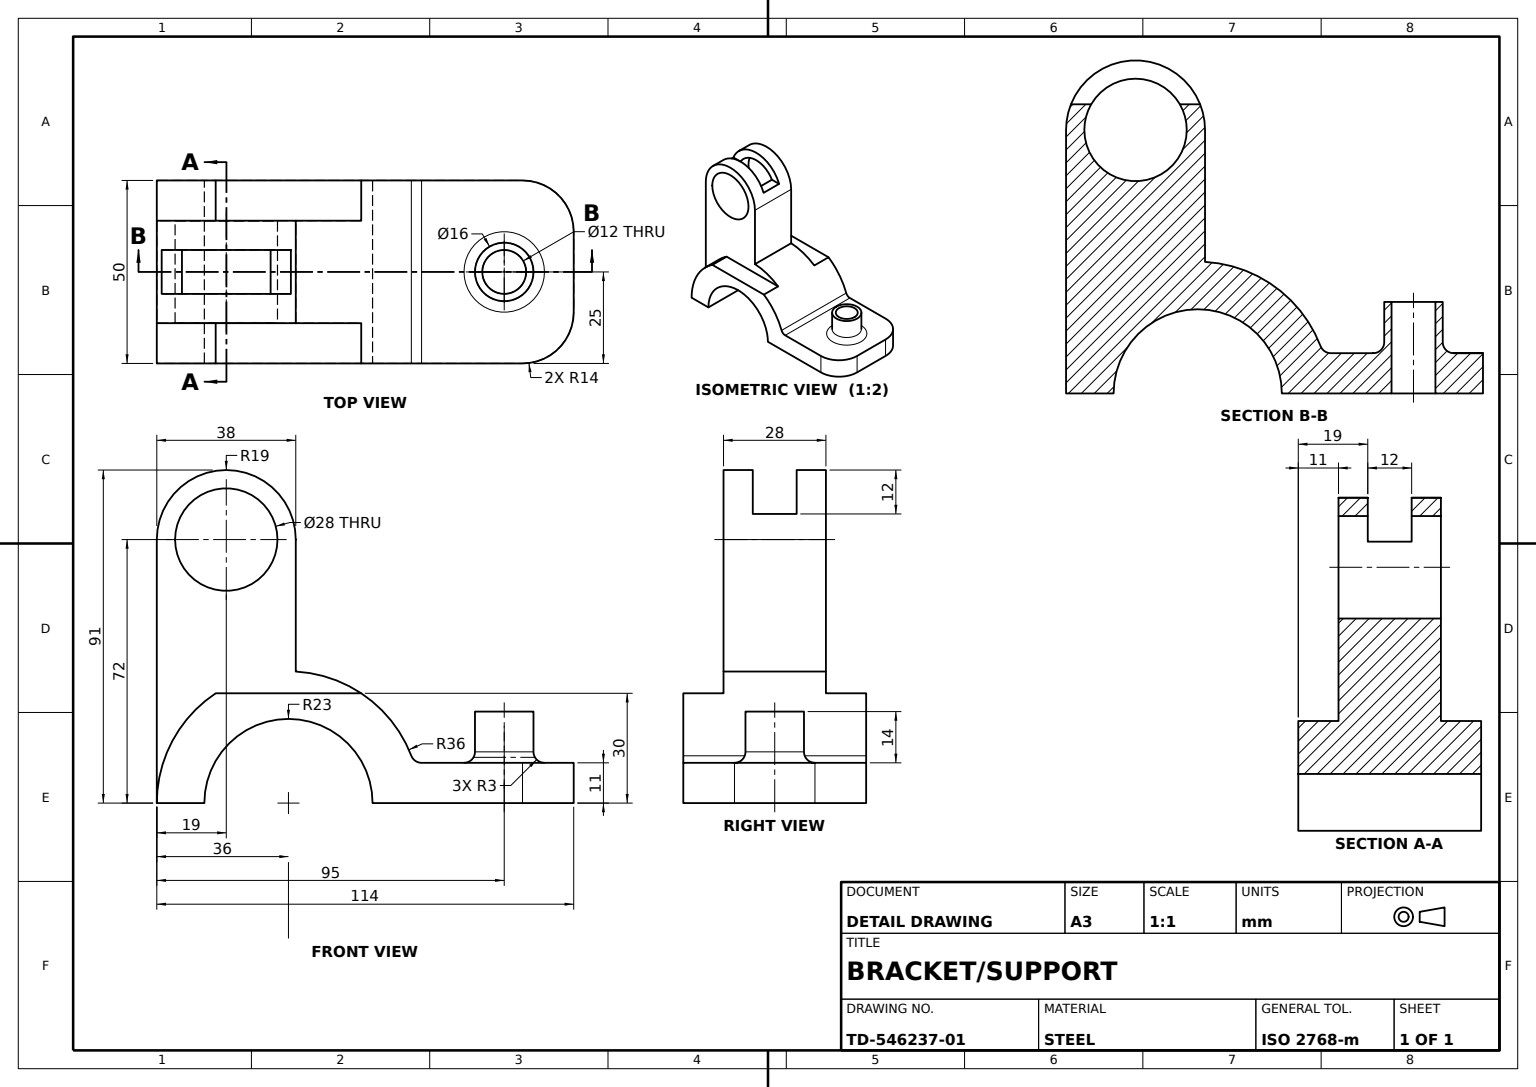
SolidWorks part; units mm, degrees
material "Plain Carbon Steel"
ref_plane "Front Plane" through (0, 0, 0) normal (0, 0, 1) x (1, 0, 0)
ref_plane "Top Plane" through (0, 0, 0) normal (0, 1, 0) x (1, 0, 0)
ref_plane "Right Plane" through (0, 0, 0) normal (1, 0, 0) x (0, 0, -1)
sketch "Base Saddle Profile Sketch" plane through (0, 0, 0) normal (1, 0, 0) x (0, 0, -1)
  line L0 (23, 0) -> (78, 0)
  line L1 (78, 0) -> (78, 11)
  line L2 (78, 11) -> (34.2783, 11)
  line L3 (23, 0) -> (-36, 0) construction
  line L5 (-23, 0) -> (-36, 0)
  arc A0 (34.2783, 11) -> (-36, 0) centre (0, 0) ccw
  arc A1 (23, 0) -> (-23, 0) centre (0, 0) ccw
  dimension "D1" = 72
  dimension "D2" = 46
  dimension "D3" = 11
  dimension "D4" = 114
extrude "Base Saddle" add sketch "Base Saddle Profile Sketch" along normal mid plane 50
fillet "Base Corner Fillet R14" radius 14 2 edges at (25, 5.5, -78) (-25, 5.5, -78)
sketch "Pin Boss Sketch" plane through (0, 11, 0) normal (0, 1, 0) x (1, 0, 0)
  line L0 (25, -36) -> (-25, -36) construction
  circle A0 centre (0, 59) radius 8
  dimension "D1" = 16
  dimension "D2" = 95
extrude "Pivot Pin Boss Ø16" add sketch "Pin Boss Sketch" along normal blind 14
sketch "Pin Boss Bore Sketch" plane through (0, 25, 0) normal (0, 1, 0) x (1, 0, 0)
  circle A0 centre (0, 59) radius 6
  dimension "D1" = 12
extrude "Pin Boss Bore Ø12" cut sketch "Pin Boss Bore Sketch" against normal through all
fillet "Pin Boss Root Fillet R3" radius 3 2 edges at (0, 11, -34.2783) (0, 11, -67)
sketch "Clevis Upright Sketch" plane through (0, 0, 0) normal (1, 0, 0) x (0, 0, -1)
  line L2 (-36, 0) -> (-36, 72)
  line L3 (-36, 72) -> (2, 72)
  line L4 (2, 35.9444) -> (2, 72)
  arc A0 (33.6005, 12.9231) -> (-36, 0) centre (0, 0) ccw construction
  arc A1 (2, 35.9444) -> (-36, 0) centre (0, 0) ccw
  dimension "D1" = 38
  dimension "D2" = 72
extrude "Clevis Upright" add sketch "Clevis Upright Sketch" along normal mid plane 28
sketch "Eye Boss Sketch" plane through (0, 0, 0) normal (1, 0, 0) x (0, 0, -1)
  line L2 (2, 72) -> (-36, 72) construction
  circle A1 centre (-17, 72) radius 19
extrude "Eye Boss" add sketch "Eye Boss Sketch" along normal mid plane 28
sketch "Eye Bore Sketch" plane through (-14, 0, 0) normal (-1, 0, 0) x (0, 0, 1)
  circle A0 centre (17, 72) radius 14
  arc A1 (36, 72) -> (-2, 72) centre (17, 72) ccw construction
  dimension "D1" = 28
extrude "Eye Bore Ø28" cut sketch "Eye Bore Sketch" against normal through all
sketch "Saddle Clearance Sketch" plane through (-25, 0, 0) normal (-1, 0, 0) x (0, 0, 1)
  line L0 (-19.8997, 30) -> (19.8997, 30)
  arc A0 (36, 0) -> (-33.6005, 12.9231) centre (0, 0) ccw construction
  arc A1 (36, 0) -> (-2, 35.9444) centre (0, 0) ccw construction
  arc A3 (-19.8997, 30) -> (19.8997, 30) centre (0, 0) cw
  dimension "D1" = 30
extrude "Saddle Clearance Cut" cut sketch "Saddle Clearance Sketch" against normal up to surface (11 mm away) up to face at (-14, 72, 31)
sketch "Saddle Relief Sketch" plane through (25, 0, 0) normal (1, 0, 0) x (0, 0, -1)
  line L0 (19.8997, 30) -> (-19.8997, 30) construction
  line L1 (19.8997, 30) -> (-19.8997, 30)
  arc A0 (-19.8997, 30) -> (19.8997, 30) centre (0, 0) cw
  arc A1 (33.6005, 12.9231) -> (-36, 0) centre (0, 0) ccw construction
extrude "Saddle Relief Cut" cut sketch "Saddle Relief Sketch" against normal up to surface (11 mm away) up to face at (14, 72, 3)
ref_plane "Clevis Top Plane" through (0, 91, 0) normal (0, -1, 0) x (-1, 0, 0)
sketch "Clevis Slot Sketch" plane through (0, 91, 0) normal (0, -1, 0) x (-1, 0, 0)
  line L0 (-14, -36) -> (14, -36) construction
  line L1 (6, 2) -> (-6, 2)
  line L2 (6, 2) -> (6, -36)
  line L3 (6, -36) -> (-6, -36)
  line L4 (-6, 2) -> (-6, -36)
  line L5 (-14, 2) -> (14, 2) construction
  point P4 (0, -36)
  dimension "D2" = 12
extrude "Clevis Slot 12" cut sketch "Clevis Slot Sketch" along normal blind 12
